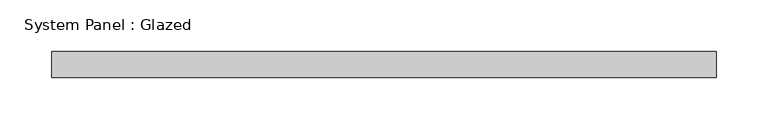
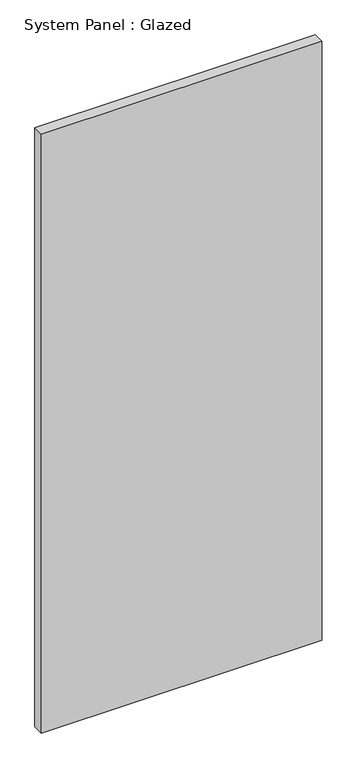
"""IFC4 building model written with IfcOpenShell, lengths in millimetres: plate geometry, System Panel : Glazed."""

from ifc_helpers import new_model, si_unit, origin, origin_with_axes, place, context, project, spatial, polyline, outline, extrude, source, transform, mapped, element, save


def system_panel_glazed_d2b782c8(model_context):
    return source(origin(), model_context, "Body", "SweptSolid", [
        extrude(outline(polyline([(322.7916667, 19.05), (-322.7916667, 19.05), (-322.7916667, 44.45), (322.7916667, 44.45), (322.7916667, 19.05)])), origin_with_axes(), (0.0, 0.0, 1.0), 1457.3599864),
    ])


if __name__ == "__main__":
    model = new_model("IFC4")
    model_context = context("Model", 3, world=origin())
    ifc_project = project(units=[si_unit("LENGTHUNIT", "METRE", prefix="MILLI")], contexts=[model_context])
    site = spatial("IfcSite", under=ifc_project)
    building = spatial("IfcBuilding", under=site)
    placement = place(None, origin())
    system_panel_glazed_shape = system_panel_glazed_d2b782c8(model_context)
    element("IfcPlate", 1, ObjectType="System Panel : Glazed", at=placement, inside=building, context=model_context, shape_type="MappedRepresentation", body=[
        mapped(system_panel_glazed_shape, transform((0.0, 0.0, 0.0), x_axis=(1.0, 0.0, 0.0), y_axis=(0.0, 1.0, 0.0), z_axis=(0.0, 0.0, 1.0))),
    ])
    save(model, "model.ifc")

# Revit data of these elements
# Type "System Panel : Glazed"
#   Construction Type Id = "GSP4R"
#   Analytic Construction = "1/8 in Pilkington single glazing"
#   Visual Light Transmittance = 0.9
#   Solar Heat Gain Coefficient = 0.86
#   Heat Transfer Coefficient (U) = 1.18115 BTU/(h·ft²·°F)
#   Define Thermal Properties by = 1
# Element 1 (IfcPlate, "System Panel : Glazed")
#   Materials on its faces: "Glass"
# Materials
#   "Glass": class "Glass", colour RGB 0 128 192, transparency 0.75, Description = "Soda Lime Glass", Cost = 0
